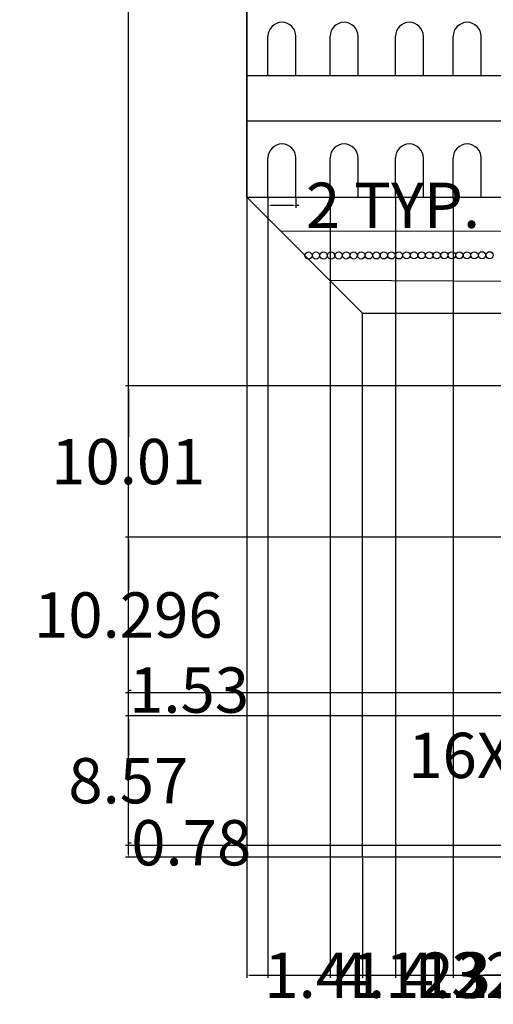
# Model space of a CAD drawing. Units: inches. Extents: x 168 to 318, y 152 to 314.
# Tile 1 of 7: x 170 to 201, y 152 to 218. Entities that reach past the tile are written whole.
import ezdxf

# ---------------------------------------------------------------- set-up
doc = ezdxf.new("R2010")
doc.units = ezdxf.units.IN
doc.header["$MEASUREMENT"] = 0
doc.layers.add('A-ANNO-DIMS', color=2, linetype='Continuous', lineweight=18)
doc.layers.add('A-ELEV', color=7, linetype='Continuous', lineweight=25)
doc.styles.get("Standard").update_dxf_attribs({"font": 'arial.ttf'})
doc.dimstyles.get("Standard").update_dxf_attribs({"dimtxt": 3, "dimasz": 0.18, "dimexe": 0.18, "dimexo": 0.0625, "dimgap": 0.09, "dimtad": 0, "dimtih": 1, "dimtoh": 1, "dimdec": 1, "dimzin": 0, "dimdsep": 46, "dimlunit": 3, "dimtxsty": 'Standard', "dimcen": 0.09, "dimadec": 0, "dimazin": 0, "dimtfac": 1, "dimtdec": 1, "dimtofl": 0, "dimtmove": 0, "dimatfit": 3, "dimfxl": 1, "dimtolj": 1, "dimtzin": 0, "dimarcsym": 0})

# ---------------------------------------------------------------- blocks, each defined once
blk = doc.blocks.new('ARCH-BALCONY-SM')
for p, q in [((0, 0), (0, 2.603)), ((1.853, 0), (1.853, 2.603))]:
    blk.add_line(p, q)
blk.add_arc((0.926, 2.603), 0.926, 0, 180)
blk = doc.blocks.new('*D12')
at = {"layer": 'A-ANNO-DIMS', "color": 0, "lineweight": -2, "ltscale": 0.2, "transparency": 16777216}
for p, q in [((186.134, 205.813), (186.134, 205.166)), ((186.314, 205.346), (187.807, 205.346)), ((187.987, 205.813), (187.987, 205.166)), ((187.987, 205.346), (188.167, 205.346))]:
    blk.add_line(p, q, dxfattribs=at)
at = {"layer": 'A-ANNO-DIMS', "color": 0, "ltscale": 0.2, "transparency": 16777216}
for points in [[(186.314, 205.376), (186.314, 205.316), (186.134, 205.346)], [(187.807, 205.376), (187.807, 205.316), (187.987, 205.346)]]:
    blk.add_solid(points, dxfattribs=at)
at = {"layer": 'Defpoints', "color": 0, "ltscale": 0.2, "transparency": 16777216}
for p in [(186.134, 205.875), (187.987, 205.875), (187.987, 205.346)]:
    blk.add_point(p, dxfattribs=at)
at = {"layer": 'A-ANNO-DIMS', "color": 0, "ltscale": 0.2, "transparency": 16777216, "insert": (194.418, 205.346), "char_height": 3, "attachment_point": 5}
blk.add_mtext('\\A1;2 TYP.', dxfattribs=at)
blk = doc.blocks.new('*D29')
at = {"layer": 'A-ANNO-DIMS', "color": 0, "lineweight": -2, "ltscale": 0.2, "transparency": 16777216}
for p, q in [((184.724, 242.139), (184.724, 154.215)), ((299.445, 242.139), (299.445, 154.215)), ((184.904, 154.395), (235.924, 154.395)), ((299.265, 154.395), (248.245, 154.395))]:
    blk.add_line(p, q, dxfattribs=at)
at = {"layer": 'A-ANNO-DIMS', "color": 0, "ltscale": 0.2, "transparency": 16777216}
for points in [[(184.904, 154.425), (184.904, 154.365), (184.724, 154.395)], [(299.265, 154.425), (299.265, 154.365), (299.445, 154.395)]]:
    blk.add_solid(points, dxfattribs=at)
at = {"layer": 'Defpoints', "color": 0, "ltscale": 0.2, "transparency": 16777216}
for p in [(184.724, 242.201), (299.445, 242.201), (299.445, 154.395)]:
    blk.add_point(p, dxfattribs=at)
at = {"layer": 'A-ANNO-DIMS', "color": 0, "ltscale": 0.2, "transparency": 16777216, "insert": (242.084, 154.395), "char_height": 3, "attachment_point": 5}
blk.add_mtext('\\A1;114.72', dxfattribs=at)
blk = doc.blocks.new('*D33')
at = {"layer": 'A-ANNO-DIMS', "color": 0, "lineweight": -2, "ltscale": 0.2, "transparency": 16777216}
for p, q in [((198.342, 304.431), (176.701, 304.431)), ((176.881, 304.251), (176.881, 234.909)), ((176.881, 162.375), (176.881, 231.717)), ((192.342, 162.195), (176.701, 162.195))]:
    blk.add_line(p, q, dxfattribs=at)
at = {"layer": 'A-ANNO-DIMS', "color": 0, "ltscale": 0.2, "transparency": 16777216}
for points in [[(176.851, 304.251), (176.911, 304.251), (176.881, 304.431)], [(176.851, 162.375), (176.911, 162.375), (176.881, 162.195)]]:
    blk.add_solid(points, dxfattribs=at)
at = {"layer": 'Defpoints', "color": 0, "ltscale": 0.2, "transparency": 16777216}
for p in [(176.881, 304.431), (198.404, 304.431), (192.404, 162.195)]:
    blk.add_point(p, dxfattribs=at)
at = {"layer": 'A-ANNO-DIMS', "color": 0, "ltscale": 0.2, "transparency": 16777216, "insert": (176.881, 233.313), "char_height": 3, "attachment_point": 5}
blk.add_mtext('\\A1;142.24', dxfattribs=at)
blk = doc.blocks.new('*D48')
at = {"layer": 'A-ANNO-DIMS', "color": 0, "lineweight": -2, "ltscale": 0.2, "transparency": 16777216}
for p, q in [((192.404, 162.133), (192.404, 154.215)), ((204.404, 162.133), (204.404, 154.215)), ((192.584, 154.395), (196.322, 154.395)), ((204.224, 154.395), (200.487, 154.395))]:
    blk.add_line(p, q, dxfattribs=at)
at = {"layer": 'A-ANNO-DIMS', "color": 0, "ltscale": 0.2, "transparency": 16777216}
for points in [[(192.584, 154.425), (192.584, 154.365), (192.404, 154.395)], [(204.224, 154.425), (204.224, 154.365), (204.404, 154.395)]]:
    blk.add_solid(points, dxfattribs=at)
at = {"layer": 'Defpoints', "color": 0, "ltscale": 0.2, "transparency": 16777216}
for p in [(192.404, 162.195), (204.404, 162.195), (204.404, 154.395)]:
    blk.add_point(p, dxfattribs=at)
at = {"layer": 'A-ANNO-DIMS', "color": 0, "ltscale": 0.2, "transparency": 16777216, "insert": (198.404, 154.395), "char_height": 3, "attachment_point": 5}
blk.add_mtext('\\A1;12', dxfattribs=at)
blk = doc.blocks.new('*D58')
at = {"layer": 'A-ANNO-DIMS', "color": 0, "lineweight": -2, "ltscale": 0.2, "transparency": 16777216}
for p, q in [((209.262, 162.979), (176.701, 162.979)), ((176.881, 162.979), (176.881, 163.159)), ((176.881, 163.159), (177.061, 163.159)), ((176.881, 162.375), (176.881, 162.799)), ((204.342, 162.195), (176.701, 162.195))]:
    blk.add_line(p, q, dxfattribs=at)
at = {"layer": 'A-ANNO-DIMS', "color": 0, "ltscale": 0.2, "transparency": 16777216}
for points in [[(176.851, 162.799), (176.911, 162.799), (176.881, 162.979)], [(176.851, 162.375), (176.911, 162.375), (176.881, 162.195)]]:
    blk.add_solid(points, dxfattribs=at)
at = {"layer": 'Defpoints', "color": 0, "ltscale": 0.2, "transparency": 16777216}
for p in [(176.881, 162.979), (209.325, 162.979), (204.404, 162.195)]:
    blk.add_point(p, dxfattribs=at)
at = {"layer": 'A-ANNO-DIMS', "color": 0, "ltscale": 0.2, "transparency": 16777216, "insert": (181.05, 163.159), "char_height": 3, "attachment_point": 5}
blk.add_mtext('\\A1;0.78', dxfattribs=at)
blk = doc.blocks.new('*D59')
at = {"layer": 'A-ANNO-DIMS', "color": 0, "lineweight": -2, "ltscale": 0.2, "transparency": 16777216}
for p, q in [((209.262, 171.549), (176.701, 171.549)), ((176.881, 171.369), (176.881, 168.886)), ((176.881, 163.159), (176.881, 165.642)), ((209.262, 162.979), (176.701, 162.979))]:
    blk.add_line(p, q, dxfattribs=at)
at = {"layer": 'A-ANNO-DIMS', "color": 0, "ltscale": 0.2, "transparency": 16777216}
for points in [[(176.851, 171.369), (176.911, 171.369), (176.881, 171.549)], [(176.851, 163.159), (176.911, 163.159), (176.881, 162.979)]]:
    blk.add_solid(points, dxfattribs=at)
at = {"layer": 'Defpoints', "color": 0, "ltscale": 0.2, "transparency": 16777216}
for p in [(176.881, 171.549), (209.325, 171.549), (209.325, 162.979)]:
    blk.add_point(p, dxfattribs=at)
at = {"layer": 'A-ANNO-DIMS', "color": 0, "ltscale": 0.2, "transparency": 16777216, "insert": (176.881, 167.264), "char_height": 3, "attachment_point": 5}
blk.add_mtext('\\A1;8.57', dxfattribs=at)
blk = doc.blocks.new('*D60')
at = {"layer": 'A-ANNO-DIMS', "color": 0, "lineweight": -2, "ltscale": 0.2, "transparency": 16777216}
for p, q in [((209.262, 173.082), (176.701, 173.082)), ((176.881, 173.082), (176.881, 173.262)), ((176.881, 173.262), (177.061, 173.262)), ((176.881, 171.729), (176.881, 172.902)), ((209.262, 171.549), (176.701, 171.549))]:
    blk.add_line(p, q, dxfattribs=at)
at = {"layer": 'A-ANNO-DIMS', "color": 0, "ltscale": 0.2, "transparency": 16777216}
for points in [[(176.851, 172.902), (176.911, 172.902), (176.881, 173.082)], [(176.851, 171.729), (176.911, 171.729), (176.881, 171.549)]]:
    blk.add_solid(points, dxfattribs=at)
at = {"layer": 'Defpoints', "color": 0, "ltscale": 0.2, "transparency": 16777216}
for p in [(176.881, 173.082), (209.325, 173.082), (209.325, 171.549)]:
    blk.add_point(p, dxfattribs=at)
at = {"layer": 'A-ANNO-DIMS', "color": 0, "ltscale": 0.2, "transparency": 16777216, "insert": (180.906, 173.262), "char_height": 3, "attachment_point": 5}
blk.add_mtext('\\A1;1.53', dxfattribs=at)
blk = doc.blocks.new('*D61')
at = {"layer": 'A-ANNO-DIMS', "color": 0, "lineweight": -2, "ltscale": 0.2, "transparency": 16777216}
for p, q in [((209.262, 183.379), (176.701, 183.379)), ((176.881, 183.199), (176.881, 179.852)), ((176.881, 173.262), (176.881, 176.609)), ((209.262, 173.082), (176.701, 173.082))]:
    blk.add_line(p, q, dxfattribs=at)
at = {"layer": 'A-ANNO-DIMS', "color": 0, "ltscale": 0.2, "transparency": 16777216}
for points in [[(176.851, 183.199), (176.911, 183.199), (176.881, 183.379)], [(176.851, 173.262), (176.911, 173.262), (176.881, 173.082)]]:
    blk.add_solid(points, dxfattribs=at)
at = {"layer": 'Defpoints', "color": 0, "ltscale": 0.2, "transparency": 16777216}
for p in [(176.881, 183.379), (209.325, 183.379), (209.325, 173.082)]:
    blk.add_point(p, dxfattribs=at)
at = {"layer": 'A-ANNO-DIMS', "color": 0, "ltscale": 0.2, "transparency": 16777216, "insert": (176.881, 178.231), "char_height": 3, "attachment_point": 5}
blk.add_mtext('\\A1;10.296', dxfattribs=at)
blk = doc.blocks.new('*D62')
at = {"layer": 'A-ANNO-DIMS', "color": 0, "lineweight": -2, "ltscale": 0.2, "transparency": 16777216}
for p, q in [((209.262, 193.388), (176.701, 193.388)), ((176.881, 193.208), (176.881, 190.005)), ((176.881, 183.559), (176.881, 186.762)), ((209.262, 183.379), (176.701, 183.379))]:
    blk.add_line(p, q, dxfattribs=at)
at = {"layer": 'A-ANNO-DIMS', "color": 0, "ltscale": 0.2, "transparency": 16777216}
for points in [[(176.851, 193.208), (176.911, 193.208), (176.881, 193.388)], [(176.851, 183.559), (176.911, 183.559), (176.881, 183.379)]]:
    blk.add_solid(points, dxfattribs=at)
at = {"layer": 'Defpoints', "color": 0, "ltscale": 0.2, "transparency": 16777216}
for p in [(176.881, 193.388), (209.325, 193.388), (209.325, 183.379)]:
    blk.add_point(p, dxfattribs=at)
at = {"layer": 'A-ANNO-DIMS', "color": 0, "ltscale": 0.2, "transparency": 16777216, "insert": (176.881, 188.383), "char_height": 3, "attachment_point": 5}
blk.add_mtext('\\A1;10.01', dxfattribs=at)
blk = doc.blocks.new('*D68')
at = {"layer": 'A-ANNO-DIMS', "color": 0, "lineweight": -2, "ltscale": 0.2, "transparency": 16777216}
for p, q in [((184.724, 205.813), (184.724, 154.215)), ((186.134, 205.813), (186.134, 154.215)), ((184.904, 154.395), (185.954, 154.395)), ((186.134, 154.395), (186.314, 154.395))]:
    blk.add_line(p, q, dxfattribs=at)
at = {"layer": 'A-ANNO-DIMS', "color": 0, "ltscale": 0.2, "transparency": 16777216}
for points in [[(184.904, 154.425), (184.904, 154.365), (184.724, 154.395)], [(185.954, 154.425), (185.954, 154.365), (186.134, 154.395)]]:
    blk.add_solid(points, dxfattribs=at)
at = {"layer": 'Defpoints', "color": 0, "ltscale": 0.2, "transparency": 16777216}
for p in [(184.724, 205.875), (186.134, 205.875), (186.134, 154.395)]:
    blk.add_point(p, dxfattribs=at)
at = {"layer": 'A-ANNO-DIMS', "color": 0, "ltscale": 0.2, "transparency": 16777216, "insert": (189.869, 154.395), "char_height": 3, "attachment_point": 5}
blk.add_mtext('\\A1;1.41', dxfattribs=at)
blk = doc.blocks.new('*D69')
at = {"layer": 'A-ANNO-DIMS', "color": 0, "lineweight": -2, "ltscale": 0.2, "transparency": 16777216}
for p, q in [((186.134, 205.813), (186.134, 154.215)), ((190.252, 205.813), (190.252, 154.215)), ((186.314, 154.395), (190.072, 154.395)), ((190.252, 154.395), (190.432, 154.395))]:
    blk.add_line(p, q, dxfattribs=at)
at = {"layer": 'A-ANNO-DIMS', "color": 0, "ltscale": 0.2, "transparency": 16777216}
for points in [[(186.314, 154.425), (186.314, 154.365), (186.134, 154.395)], [(190.072, 154.425), (190.072, 154.365), (190.252, 154.395)]]:
    blk.add_solid(points, dxfattribs=at)
at = {"layer": 'Defpoints', "color": 0, "ltscale": 0.2, "transparency": 16777216}
for p in [(186.134, 205.875), (190.252, 205.875), (190.252, 154.395)]:
    blk.add_point(p, dxfattribs=at)
at = {"layer": 'A-ANNO-DIMS', "color": 0, "ltscale": 0.2, "transparency": 16777216, "insert": (194.464, 154.395), "char_height": 3, "attachment_point": 5}
blk.add_mtext('\\A1;4.12', dxfattribs=at)
blk = doc.blocks.new('*D70')
at = {"layer": 'A-ANNO-DIMS', "color": 0, "lineweight": -2, "ltscale": 0.2, "transparency": 16777216}
for p, q in [((190.252, 205.813), (190.252, 154.215)), ((194.576, 205.813), (194.576, 154.215)), ((190.432, 154.395), (194.396, 154.395)), ((194.576, 154.395), (194.756, 154.395))]:
    blk.add_line(p, q, dxfattribs=at)
at = {"layer": 'A-ANNO-DIMS', "color": 0, "ltscale": 0.2, "transparency": 16777216}
for points in [[(190.432, 154.425), (190.432, 154.365), (190.252, 154.395)], [(194.396, 154.425), (194.396, 154.365), (194.576, 154.395)]]:
    blk.add_solid(points, dxfattribs=at)
at = {"layer": 'Defpoints', "color": 0, "ltscale": 0.2, "transparency": 16777216}
for p in [(190.252, 205.875), (194.576, 205.875), (194.576, 154.395)]:
    blk.add_point(p, dxfattribs=at)
at = {"layer": 'A-ANNO-DIMS', "color": 0, "ltscale": 0.2, "transparency": 16777216, "insert": (199.968, 154.395), "char_height": 3, "attachment_point": 5}
blk.add_mtext('\\A1;4.323', dxfattribs=at)
blk = doc.blocks.new('*D71')
at = {"layer": 'A-ANNO-DIMS', "color": 0, "lineweight": -2, "ltscale": 0.2, "transparency": 16777216}
for p, q in [((194.576, 205.813), (194.576, 154.215)), ((198.404, 205.813), (198.404, 154.215)), ((194.756, 154.395), (198.224, 154.395)), ((198.404, 154.395), (198.584, 154.395))]:
    blk.add_line(p, q, dxfattribs=at)
at = {"layer": 'A-ANNO-DIMS', "color": 0, "ltscale": 0.2, "transparency": 16777216}
for points in [[(194.756, 154.425), (194.756, 154.365), (194.576, 154.395)], [(198.224, 154.425), (198.224, 154.365), (198.404, 154.395)]]:
    blk.add_solid(points, dxfattribs=at)
at = {"layer": 'Defpoints', "color": 0, "ltscale": 0.2, "transparency": 16777216}
for p in [(194.576, 205.875), (198.404, 205.875), (198.404, 154.395)]:
    blk.add_point(p, dxfattribs=at)
at = {"layer": 'A-ANNO-DIMS', "color": 0, "ltscale": 0.2, "transparency": 16777216, "insert": (203.738, 154.395), "char_height": 3, "attachment_point": 5}
blk.add_mtext('\\A1;3.829', dxfattribs=at)
blk = doc.blocks.new('*D72')
at = {"layer": 'A-ANNO-DIMS', "color": 0, "lineweight": -2, "ltscale": 0.2, "transparency": 16777216}
for p, q in [((198.404, 205.813), (198.404, 154.215)), ((202.463, 205.813), (202.463, 154.215)), ((198.584, 154.395), (202.283, 154.395)), ((202.463, 154.395), (202.643, 154.395))]:
    blk.add_line(p, q, dxfattribs=at)
at = {"layer": 'A-ANNO-DIMS', "color": 0, "ltscale": 0.2, "transparency": 16777216}
for points in [[(198.584, 154.425), (198.584, 154.365), (198.404, 154.395)], [(202.283, 154.425), (202.283, 154.365), (202.463, 154.395)]]:
    blk.add_solid(points, dxfattribs=at)
at = {"layer": 'Defpoints', "color": 0, "ltscale": 0.2, "transparency": 16777216}
for p in [(198.404, 205.875), (202.463, 205.875), (202.463, 154.395)]:
    blk.add_point(p, dxfattribs=at)
at = {"layer": 'A-ANNO-DIMS', "color": 0, "ltscale": 0.2, "transparency": 16777216, "insert": (207.858, 154.395), "char_height": 3, "attachment_point": 5}
blk.add_mtext('\\A1;4.058', dxfattribs=at)
blk = doc.blocks.new('*D100')
at = {"layer": 'A-ANNO-DIMS', "color": 0, "lineweight": -2, "ltscale": 0.2, "transparency": 16777216}
for p, q in [((208.521, 168.938), (208.701, 168.938)), ((208.701, 168.938), (210.193, 168.308)), ((213.033, 167.072), (213.213, 167.072)), ((213.123, 166.982), (213.123, 167.162))]:
    blk.add_line(p, q, dxfattribs=at)
at = {"layer": 'A-ANNO-DIMS', "color": 0, "ltscale": 0.2, "transparency": 16777216}
blk.add_solid([(210.205, 168.336), (210.182, 168.28), (210.359, 168.238)], dxfattribs=at)
at = {"layer": 'Defpoints', "color": 0, "ltscale": 0.2, "transparency": 16777216}
for p in [(210.359, 168.238), (213.123, 167.072)]:
    blk.add_point(p, dxfattribs=at)
at = {"layer": 'A-ANNO-DIMS', "color": 0, "ltscale": 0.2, "transparency": 16777216, "insert": (201.765, 168.938), "char_height": 3, "attachment_point": 5}
blk.add_mtext('\\A1;16X R3', dxfattribs=at)

msp = doc.modelspace()

# ---------------------------------------------------------------- linework, layer by layer
at = {"layer": 'A-ELEV'}
for p, q in [((184.7244, 205.8755), (184.7244, 220.8755)), ((184.7244, 213.9241), (212.0845, 213.9241)), ((184.7244, 210.9241), (212.0845, 210.9241)), ((192.4044, 198.1954), (184.7244, 205.8755)), ((184.7244, 205.8755), (212.0845, 205.8755)), ((186.9522, 203.6477), (209.8404, 203.6314)), ((190.2158, 200.3841), (206.511, 200.302)), ((192.4044, 162.1954), (192.4044, 198.1954)), ((192.4044, 198.1954), (204.4044, 198.1954)), ((204.4044, 162.1954), (192.4044, 162.1954))]:
    msp.add_line(p, q, dxfattribs=at)
for centre in [(188.8149, 202.0204), (189.3149, 202.0211), (189.8149, 202.0218), (190.3149, 202.0225), (190.8149, 202.0232), (191.3149, 202.024), (191.8149, 202.0247), (192.3149, 202.0254), (192.8149, 202.0261), (193.3149, 202.0268), (193.8149, 202.0275), (194.3149, 202.0283), (194.8149, 202.029), (195.3149, 202.0297), (195.8149, 202.0304), (196.3149, 202.0311), (196.8149, 202.0318), (197.3149, 202.0326), (197.8149, 202.0333), (198.3149, 202.034), (198.8149, 202.0347), (199.3149, 202.0354), (199.8149, 202.0361), (200.3149, 202.0369), (200.8149, 202.0376)]:
    msp.add_circle(centre, 0.2354, dxfattribs=at)

# ---------------------------------------------------------------- block references
for p in [(186.134, 213.9237), (190.2525, 213.9237), (194.5757, 213.9237), (198.4045, 213.9237), (186.134, 205.875), (190.2525, 205.875), (194.5757, 205.875), (198.4045, 205.875)]:
    msp.add_blockref('ARCH-BALCONY-SM', p, dxfattribs=at)

# ---------------------------------------------------------------- dimensions: what is measured, and where the dimension line sits
at = {"layer": 'A-ANNO-DIMS', "ltscale": 0.2}
for base, p1, p2, override, picture, middle in [((176.8805, 304.4308), (192.4044, 162.1954), (198.4044, 304.4308), {"dimdec": 2, "dimlfac": 1, "dimrnd": 0, "dimzin": 0, "dimdsep": 46, "dimlunit": 2}, '*D33', (176.8805, 233.3131)), ((176.8805, 193.3878), (209.3248, 183.3788), (209.3248, 193.3878), {"dimdec": 2, "dimlfac": 1, "dimrnd": 0, "dimzin": 0, "dimdsep": 46, "dimlunit": 2}, '*D62', (176.8805, 188.3833)), ((176.8805, 183.3788), (209.3248, 173.0824), (209.3248, 183.3788), {"dimdec": 3, "dimlfac": 1, "dimrnd": 0, "dimzin": 0, "dimdsep": 46, "dimlunit": 2}, '*D61', (176.8805, 178.2306)), ((176.8805, 173.0824), (209.3248, 171.5491), (209.3248, 173.0824), {"dimdec": 2, "dimlfac": 1, "dimrnd": 0, "dimzin": 0, "dimdsep": 46, "dimlunit": 2}, '*D60', (180.9056, 173.2624)), ((176.8805, 171.5491), (209.3248, 162.9789), (209.3248, 171.5491), {"dimdec": 2, "dimlfac": 1, "dimrnd": 0, "dimzin": 0, "dimdsep": 46, "dimlunit": 2}, '*D59', (176.8805, 167.264)), ((176.8805, 162.9789), (204.4044, 162.1954), (209.3248, 162.9789), {"dimdec": 2, "dimlfac": 1, "dimrnd": 0, "dimzin": 0, "dimdsep": 46, "dimlunit": 2}, '*D58', (181.0499, 163.1589))]:
    dim = msp.add_linear_dim(base=base, p1=p1, p2=p2, angle=90, dimstyle='Standard', override=override, dxfattribs=at)
    dim.commit()
    dim.dimension.update_dxf_attribs({"geometry": picture, "text_midpoint": middle})
for base, p1, p2, override, picture, middle in [((299.4446, 154.3954), (184.7244, 242.2013), (299.4446, 242.2013), {"dimdec": 2, "dimlfac": 1, "dimrnd": 0, "dimzin": 0, "dimdsep": 46, "dimlunit": 2}, '*D29', (242.0845, 154.3954)), ((186.1339, 154.3954), (184.7244, 205.8755), (186.1339, 205.8755), {"dimdec": 2, "dimlfac": 1, "dimrnd": 0, "dimzin": 0, "dimdsep": 46, "dimlunit": 2}, '*D68', (189.8695, 154.3954)), ((190.2524, 154.3954), (186.1339, 205.8755), (190.2524, 205.8755), {"dimdec": 2, "dimlfac": 1, "dimrnd": 0, "dimzin": 0, "dimdsep": 46, "dimlunit": 2}, '*D69', (194.4638, 154.3954)), ((194.5757, 154.3954), (190.2524, 205.8755), (194.5757, 205.8755), {"dimdec": 3, "dimlfac": 1, "dimrnd": 0, "dimzin": 0, "dimdsep": 46, "dimlunit": 2}, '*D70', (199.9678, 154.3954)), ((198.4044, 154.3954), (194.5757, 205.8755), (198.4044, 205.8755), {"dimdec": 3, "dimlfac": 1, "dimrnd": 0, "dimzin": 0, "dimdsep": 46, "dimlunit": 2}, '*D71', (203.7382, 154.3954)), ((202.4627, 154.3954), (198.4044, 205.8755), (202.4627, 205.8755), {"dimdec": 3, "dimlfac": 1, "dimrnd": 0, "dimzin": 0, "dimdsep": 46, "dimlunit": 2}, '*D72', (207.8578, 154.3954)), ((204.4044, 154.3954), (192.4044, 162.1954), (204.4044, 162.1954), {"dimdec": 0, "dimlfac": 1, "dimrnd": 0, "dimzin": 0, "dimdsep": 46, "dimlunit": 2}, '*D48', (198.4044, 154.3954))]:
    dim = msp.add_linear_dim(base=base, p1=p1, p2=p2, dimstyle='Standard', override=override, dxfattribs=at)
    dim.commit()
    dim.dimension.update_dxf_attribs({"geometry": picture, "text_midpoint": middle})
dim = msp.add_linear_dim(base=(187.9867, 205.3462), p1=(186.1339, 205.8755), p2=(187.9867, 205.8755), text='<> TYP.', dimstyle='Standard', override={"dimdec": 0, "dimrnd": 0, "dimzin": 0, "dimlunit": 2}, dxfattribs=at)
dim.commit()
dim.dimension.update_dxf_attribs({"geometry": '*D12', "text_midpoint": (194.4183, 205.3462)})
dim = msp.add_radius_dim(center=(213.1231, 167.0717), mpoint=(210.3591, 168.238), text='16X <>', dimstyle='Standard', override={"dimdec": 0, "dimlfac": 1, "dimrnd": 0, "dimzin": 0, "dimdsep": 46, "dimlunit": 2}, dxfattribs=at)
dim.commit()
dim.dimension.update_dxf_attribs({"geometry": '*D100', "text_midpoint": (201.7646, 168.9377), "dimtype": 164})

doc.saveas('drawing.dxf')
